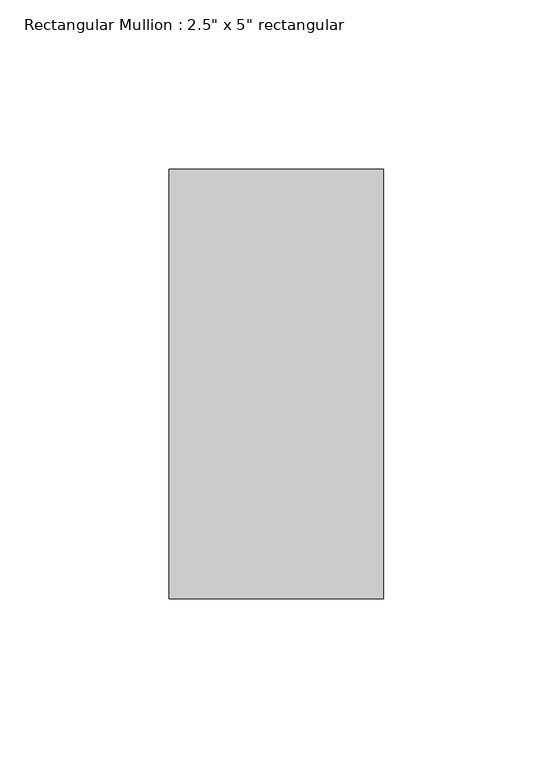
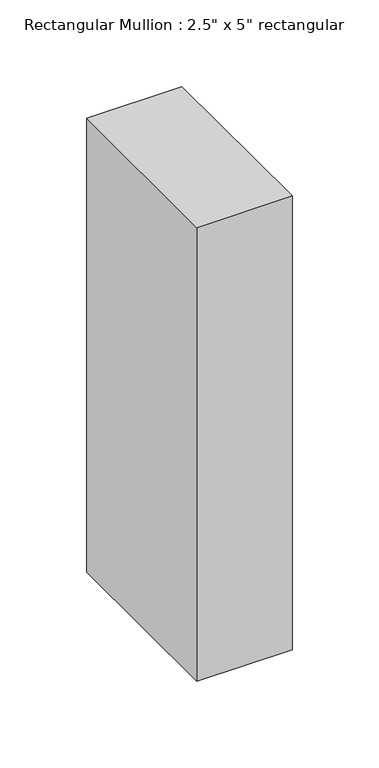
"""IFC4 building model written with IfcOpenShell, lengths in millimetres: member geometry."""

from ifc_helpers import new_model, si_unit, frame, origin, place, context, project, spatial, polyline, outline, extrude, source, transform, mapped, element, save


def member_91b02dc0(model_context):
    return source(origin(), model_context, "Body", "SweptSolid", [
        extrude(outline(polyline([(0.0, 63.5), (0.0, -63.5), (-63.5, -63.5), (-63.5, 63.5), (0.0, 63.5)])), frame((0.0, 0.0, -319.6166667), z_axis=(0.0, 0.0, 1.0), x_axis=(1.0, 0.0, 0.0)), (0.0, 0.0, 1.0), 319.6166667),
    ])


if __name__ == "__main__":
    model = new_model("IFC4")
    model_context = context("Model", 3, world=origin())
    ifc_project = project(units=[si_unit("LENGTHUNIT", "METRE", prefix="MILLI")], contexts=[model_context])
    site = spatial("IfcSite", under=ifc_project)
    building = spatial("IfcBuilding", under=site)
    placement = place(None, origin())
    member_shape = member_91b02dc0(model_context)
    element("IfcMember", 1, ObjectType="Rectangular Mullion : 2.5\" x 5\" rectangular", at=placement, inside=building, context=model_context, shape_type="MappedRepresentation", body=[
        mapped(member_shape, transform((0.0, 0.0, 0.0), x_axis=(1.0, 0.0, 0.0), y_axis=(0.0, 1.0, 0.0), z_axis=(0.0, 0.0, 1.0))),
    ])
    save(model, "model.ifc")

# Revit data of these elements
# Type "Rectangular Mullion : 2.5\" x 5\" rectangular"
#   built-in parameter 1007304 = 0.416667 (stored number, unit not read)
#   built-in parameter 1007301 = 0.104167 (stored number, unit not read)
#   built-in parameter 1007300 = 0.104167 (stored number, unit not read)
